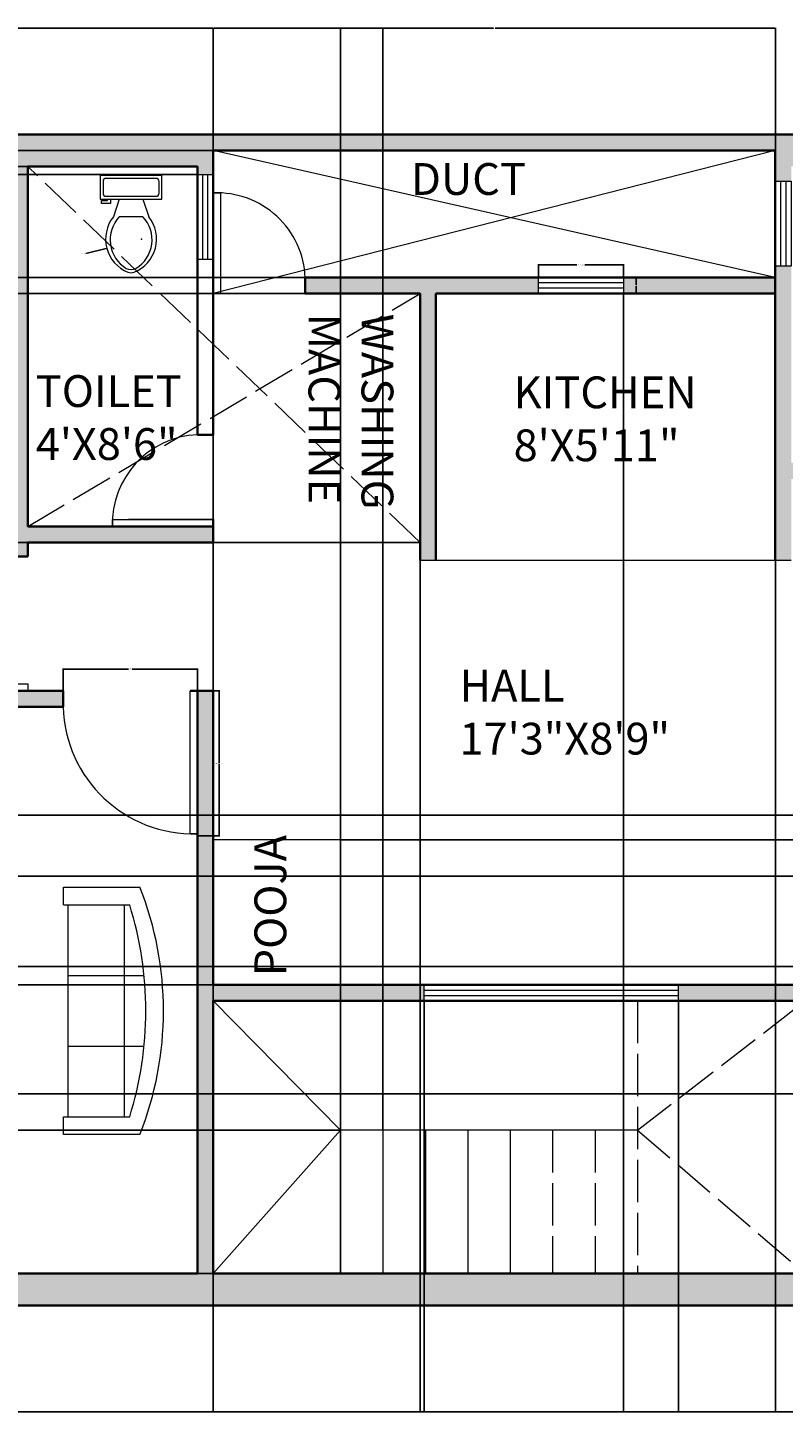
# Model space of a CAD drawing. Units: feet. Extents: x 1699 to 2359, y 1819 to 2211.
# Tile 2 of 4: x 1903 to 2117, y 1819 to 2211. Entities that reach past the tile are written whole.
import ezdxf

# ---------------------------------------------------------------- set-up
doc = ezdxf.new("R2010")
doc.units = ezdxf.units.FT
doc.linetypes.add('ACAD_ISO02W100', pattern=[15, 12, -3])
for name, color, linetype, lineweight in [('A-ANNO-DIMS', 2, 'Continuous', 18), ('A-ANNO-TEXT', 7, 'Continuous', 18), ('A-AREA-IDEN', 7, 'Continuous', 18), ('A-DOOR', 4, 'Continuous', 18), ('A-FLOR', 7, 'Continuous', 18), ('A-FLOR-FIXT', 9, 'Continuous', 18), ('A-FLOR-OVHD', 8, 'ACAD_ISO02W100', 13), ('A-FLOR-STRS', 7, 'Continuous', 18), ('A-FLOR-STRS-OVHD', 8, 'ACAD_ISO02W100', 13), ('A-FURN', 8, 'Continuous', 18), ('A-GLAZ', 3, 'Continuous', 18), ('A-WALL', 7, 'Continuous', 35), ('A-WALL-PATT', 1, 'Continuous', 13)]:
    doc.layers.add(name, color=color, linetype=linetype, lineweight=lineweight)
doc.styles.get("Standard").update_dxf_attribs({"font": 'arial.ttf'})
doc.dimstyles.get("Standard").update_dxf_attribs({"dimtxt": 0.18, "dimasz": 0.18, "dimexe": 0.18, "dimexo": 0.0625, "dimgap": 0.09, "dimtad": 0, "dimtih": 1, "dimtoh": 1, "dimdec": 4, "dimzin": 0, "dimdsep": 46, "dimtxsty": 'Standard', "dimcen": 0.09, "dimadec": 0, "dimazin": 0, "dimtfac": 1, "dimtdec": 4, "dimtofl": 0, "dimtmove": 0, "dimatfit": 3, "dimfxl": 1, "dimtolj": 1, "dimtzin": 0, "dimarcsym": 0})

# ---------------------------------------------------------------- blocks, each defined once
blk = doc.blocks.new('Toilet - top')
for p, q in [((9.5, -6), (9.5, -2)), ((-10, -8.5), (-8, -8.5)), ((-10, -9.5), (-10, -8.5)), ((-8, -8.5), (-8, -8)), ((-7, -8), (-7, -9.5)), ((-4, -8), (-6, -14)), ((4, -8), (6, -14)), ((-7, -9.5), (-10, -9.5)), ((4, -14), (-4, -14))]:
    blk.add_line(p, q)
blk.add_lwpolyline([(10.5, -8), (10.5, 0), (-10.5, 0), (-10.5, -8)], close=True)
for points in [[(-9.5, -2), (-9.5, -6)], [(8.5, -1), (-8.5, -1)], [(-8.5, -7), (8.5, -7)]]:
    blk.add_lwpolyline(points)
for centre, radius, start, end in [((-8.62, -1.88), 0.884, 81.8699, 188.1301), ((8.62, -1.88), 0.884, 351.8699, 98.1301), ((-8.62, -6.12), 0.884, 171.8699, 278.1301), ((8.62, -6.12), 0.884, 261.8699, 8.1301), ((3.52, -21.58), 12.17, 141.4691, 247.9714), ((4.2, -21.82), 11.33, 136.3677, 238.9468), ((-3.52, -21.58), 12.17, 292.0284, 38.5307), ((-4.2, -21.82), 11.33, 301.053, 43.6321), ((0, -27.88), 4, 245.7318, 294.2682), ((0, -29), 4, 254.8605, 285.1395)]:
    blk.add_arc(centre, radius, start, end)
blk = doc.blocks.new('Sofa - Roundback 7 ft.')
for p, q in [((-12.00002, -32.4421), (-12.00003, -6.5971)), ((11.99997, -32.4421), (11.99998, -6.5971)), ((-36.000027, -34), (-36.000027, -11.4696)), ((-35.999844, -13.3819), (35.9998, -13.3819)), ((35.99998, -34), (35.99998, -11.4696)), ((-36.000027, -32.4421), (35.99998, -32.4421))]:
    blk.add_line(p, q)
for points in [[(-36.000027, -34), (-42.000027, -34), (-42.000027, -8)], [(41.99998, -8), (41.99998, -34), (35.99998, -34)]]:
    blk.add_lwpolyline(points)
for centre, radius, start, end in [((0, -114.25), 114.25, 68.43141, 111.5686), ((-0.00001, -127.1968), 121.1968, 72.72033, 107.2797)]:
    blk.add_arc(centre, radius, start, end)
blk = doc.blocks.new('WIN-24-PARTITION')
for p, q in [((0, 24), (4.5, 24)), ((0, 0), (0, 24)), ((1.5, 0), (1.5, 24)), ((3, 0), (3, 24)), ((4.5, 24), (4.5, 0)), ((4.5, 0), (0, 0))]:
    blk.add_line(p, q)
blk = doc.blocks.new('DOOR-SWING-36')
for p, q in [((0.01, 0), (0.01, 2)), ((0.01, 2), (40.51, 2)), ((36.01, 0), (0.01, 0))]:
    blk.add_line(p, q)
blk.add_arc((37.01, 1), 37.01, 91.5482, 181.5482)
blk = doc.blocks.new('DOOR-SWING-24')
for p, q in [((0.02, 0), (0.02, 2)), ((0.02, 2), (28.52, 2)), ((24.02, 0), (0.02, 0))]:
    blk.add_line(p, q)
blk.add_arc((25.02, 1), 25.02, 92.2906, 182.2906)
blk = doc.blocks.new('*D16')
at = {"layer": 'A-ANNO-DIMS', "color": 0, "lineweight": -2, "transparency": 16777216}
for p, q in [((2047.43, 2139.91), (2047.43, 2143.63)), ((2047.61, 2143.45), (2058.31, 2143.45)), ((2071.25, 2143.45), (2060.55, 2143.45)), ((2071.43, 2139.91), (2071.43, 2143.63))]:
    blk.add_line(p, q, dxfattribs=at)
at = {"layer": 'A-ANNO-DIMS', "color": 0, "transparency": 16777216}
for points in [[(2047.61, 2143.48), (2047.61, 2143.42), (2047.43, 2143.45)], [(2071.25, 2143.48), (2071.25, 2143.42), (2071.43, 2143.45)]]:
    blk.add_solid(points, dxfattribs=at)
at = {"layer": 'Defpoints', "color": 0, "transparency": 16777216}
for p in [(2047.43, 2143.45), (2047.43, 2139.85), (2071.43, 2139.85)]:
    blk.add_point(p, dxfattribs=at)
at = {"layer": 'A-ANNO-DIMS', "color": 0, "transparency": 16777216, "insert": (2059.43, 2143.45), "char_height": 0.18, "attachment_point": 5}
blk.add_mtext('\\A1;WINDOW 24 TYP.', dxfattribs=at)
blk = doc.blocks.new('*D17')
at = {"layer": 'A-ANNO-DIMS', "color": 0, "lineweight": -2, "transparency": 16777216}
for p, q in [((2071.49, 2139.85), (2075.21, 2139.85)), ((2075.03, 2139.67), (2075.03, 2137.78)), ((2075.03, 2135.53), (2075.03, 2137.42)), ((2071.49, 2135.35), (2075.21, 2135.35))]:
    blk.add_line(p, q, dxfattribs=at)
at = {"layer": 'A-ANNO-DIMS', "color": 0, "transparency": 16777216}
for points in [[(2075, 2139.67), (2075.06, 2139.67), (2075.03, 2139.85)], [(2075, 2135.53), (2075.06, 2135.53), (2075.03, 2135.35)]]:
    blk.add_solid(points, dxfattribs=at)
at = {"layer": 'Defpoints', "color": 0, "transparency": 16777216}
for p in [(2071.43, 2139.85), (2075.03, 2139.85), (2071.43, 2135.35)]:
    blk.add_point(p, dxfattribs=at)
at = {"layer": 'A-ANNO-DIMS', "color": 0, "transparency": 16777216, "insert": (2075.03, 2137.6), "char_height": 0.18, "attachment_point": 5}
blk.add_mtext('\\A1;5 TYP.', dxfattribs=at)
blk = doc.blocks.new('*D20')
at = {"layer": 'A-ANNO-DIMS', "color": 0, "lineweight": -2, "transparency": 16777216}
for p, q in [((1950.99, 2022.85), (1957.26, 2022.85)), ((1957.08, 2022.67), (1957.08, 2002.51)), ((1957.08, 1981.98), (1957.08, 2002.14)), ((1950.99, 1981.8), (1957.26, 1981.8))]:
    blk.add_line(p, q, dxfattribs=at)
at = {"layer": 'A-ANNO-DIMS', "color": 0, "transparency": 16777216}
for points in [[(1957.05, 2022.67), (1957.11, 2022.67), (1957.08, 2022.85)], [(1957.05, 1981.98), (1957.11, 1981.98), (1957.08, 1981.8)]]:
    blk.add_solid(points, dxfattribs=at)
at = {"layer": 'Defpoints', "color": 0, "transparency": 16777216}
for p in [(1950.93, 2022.85), (1957.08, 2022.85), (1950.93, 1981.8)]:
    blk.add_point(p, dxfattribs=at)
at = {"layer": 'A-ANNO-DIMS', "color": 0, "transparency": 16777216, "insert": (1957.08, 2002.32), "char_height": 0.18, "attachment_point": 5}
blk.add_mtext('\\A1;DOOR D2 41 TYP.', dxfattribs=at)
blk = doc.blocks.new('*D21')
at = {"layer": 'A-ANNO-DIMS', "color": 0, "lineweight": -2, "transparency": 16777216}
for p, q in [((1912.93, 2022.91), (1912.93, 2029.19)), ((1913.11, 2029.01), (1931.4, 2029.01)), ((1950.75, 2029.01), (1932.45, 2029.01)), ((1950.93, 2022.91), (1950.93, 2029.19))]:
    blk.add_line(p, q, dxfattribs=at)
at = {"layer": 'A-ANNO-DIMS', "color": 0, "transparency": 16777216}
for points in [[(1913.11, 2029.04), (1913.11, 2028.98), (1912.93, 2029.01)], [(1950.75, 2029.04), (1950.75, 2028.98), (1950.93, 2029.01)]]:
    blk.add_solid(points, dxfattribs=at)
at = {"layer": 'Defpoints', "color": 0, "transparency": 16777216}
for p in [(1912.93, 2029.01), (1912.93, 2022.85), (1950.93, 2022.85)]:
    blk.add_point(p, dxfattribs=at)
at = {"layer": 'A-ANNO-DIMS', "color": 0, "transparency": 16777216, "insert": (1931.93, 2029.01), "char_height": 0.18, "attachment_point": 5}
blk.add_mtext('\\A1;38 TYP.', dxfattribs=at)
blk = doc.blocks.new('*D23')
at = {"layer": 'A-ANNO-DIMS', "color": 0, "lineweight": -2, "transparency": 16777216}
for p, q in [((1955.43, 1857.79), (1955.43, 1818.57)), ((2180.43, 1857.79), (2180.43, 1818.57)), ((1955.61, 1818.75), (2067.64, 1818.75)), ((2180.25, 1818.75), (2068.22, 1818.75))]:
    blk.add_line(p, q, dxfattribs=at)
at = {"layer": 'A-ANNO-DIMS', "color": 0, "transparency": 16777216}
for points in [[(1955.61, 1818.78), (1955.61, 1818.72), (1955.43, 1818.75)], [(2180.25, 1818.78), (2180.25, 1818.72), (2180.43, 1818.75)]]:
    blk.add_solid(points, dxfattribs=at)
at = {"layer": 'Defpoints', "color": 0, "transparency": 16777216}
for p in [(1955.43, 1857.85), (2180.43, 1857.85), (2180.43, 1818.75)]:
    blk.add_point(p, dxfattribs=at)
at = {"layer": 'A-ANNO-DIMS', "color": 0, "transparency": 16777216, "insert": (2067.93, 1818.75), "char_height": 0.18, "attachment_point": 5}
blk.add_mtext('\\A1;225', dxfattribs=at)
blk = doc.blocks.new('*D24')
at = {"layer": 'A-ANNO-DIMS', "color": 0, "lineweight": -2, "transparency": 16777216}
for p, q in [((1955.49, 1935.08), (2359.21, 1935.08)), ((2359.03, 1934.9), (2359.03, 1896.65)), ((2359.03, 1858.03), (2359.03, 1896.28)), ((1955.49, 1857.85), (2359.21, 1857.85))]:
    blk.add_line(p, q, dxfattribs=at)
at = {"layer": 'A-ANNO-DIMS', "color": 0, "transparency": 16777216}
for points in [[(2359, 1934.9), (2359.06, 1934.9), (2359.03, 1935.08)], [(2359, 1858.03), (2359.06, 1858.03), (2359.03, 1857.85)]]:
    blk.add_solid(points, dxfattribs=at)
at = {"layer": 'Defpoints', "color": 0, "transparency": 16777216}
for p in [(1955.43, 1935.08), (2359.03, 1935.08), (1955.43, 1857.85)]:
    blk.add_point(p, dxfattribs=at)
at = {"layer": 'A-ANNO-DIMS', "color": 0, "transparency": 16777216, "insert": (2359.03, 1896.46), "char_height": 0.18, "attachment_point": 5}
blk.add_mtext('\\A1;77.23', dxfattribs=at)
blk = doc.blocks.new('*D26')
at = {"layer": 'A-ANNO-DIMS', "color": 0, "lineweight": -2, "transparency": 16777216}
for p, q in [((1955.43, 2175.91), (1955.43, 2210.63)), ((1955.61, 2210.45), (2034.65, 2210.45)), ((2114.25, 2210.45), (2035.21, 2210.45)), ((2114.43, 2175.91), (2114.43, 2210.63))]:
    blk.add_line(p, q, dxfattribs=at)
at = {"layer": 'A-ANNO-DIMS', "color": 0, "transparency": 16777216}
for points in [[(1955.61, 2210.48), (1955.61, 2210.42), (1955.43, 2210.45)], [(2114.25, 2210.48), (2114.25, 2210.42), (2114.43, 2210.45)]]:
    blk.add_solid(points, dxfattribs=at)
at = {"layer": 'Defpoints', "color": 0, "transparency": 16777216}
for p in [(2114.43, 2210.45), (1955.43, 2175.85), (2114.43, 2175.85)]:
    blk.add_point(p, dxfattribs=at)
at = {"layer": 'A-ANNO-DIMS', "color": 0, "transparency": 16777216, "insert": (2034.93, 2210.45), "char_height": 0.18, "attachment_point": 5}
blk.add_mtext('\\A1;159', dxfattribs=at)
blk = doc.blocks.new('*D27')
at = {"layer": 'A-ANNO-DIMS', "color": 0, "lineweight": -2, "transparency": 16777216}
for p, q in [((2114.36, 2175.85), (1699.15, 2175.85)), ((1699.33, 2175.67), (1699.33, 2158.03)), ((1699.33, 2140.03), (1699.33, 2157.67)), ((2114.36, 2139.85), (1699.15, 2139.85))]:
    blk.add_line(p, q, dxfattribs=at)
at = {"layer": 'A-ANNO-DIMS', "color": 0, "transparency": 16777216}
for points in [[(1699.3, 2175.67), (1699.36, 2175.67), (1699.33, 2175.85)], [(1699.3, 2140.03), (1699.36, 2140.03), (1699.33, 2139.85)]]:
    blk.add_solid(points, dxfattribs=at)
at = {"layer": 'Defpoints', "color": 0, "transparency": 16777216}
for p in [(2114.43, 2175.85), (1699.33, 2139.85), (2114.43, 2139.85)]:
    blk.add_point(p, dxfattribs=at)
at = {"layer": 'A-ANNO-DIMS', "color": 0, "transparency": 16777216, "insert": (1699.33, 2157.85), "char_height": 0.18, "attachment_point": 5}
blk.add_mtext('\\A1;36', dxfattribs=at)
blk = doc.blocks.new('*D30')
at = {"layer": 'A-ANNO-DIMS', "color": 0, "lineweight": -2, "transparency": 16777216}
for p, q in [((1955.43, 1935.02), (1955.43, 1818.57)), ((2015.05, 1935.02), (2015.05, 1818.57)), ((1955.61, 1818.75), (1984.85, 1818.75)), ((2014.87, 1818.75), (1985.63, 1818.75))]:
    blk.add_line(p, q, dxfattribs=at)
at = {"layer": 'A-ANNO-DIMS', "color": 0, "transparency": 16777216}
for points in [[(1955.61, 1818.78), (1955.61, 1818.72), (1955.43, 1818.75)], [(2014.87, 1818.78), (2014.87, 1818.72), (2015.05, 1818.75)]]:
    blk.add_solid(points, dxfattribs=at)
at = {"layer": 'Defpoints', "color": 0, "transparency": 16777216}
for p in [(1955.43, 1935.08), (2015.05, 1935.08), (2015.05, 1818.75)]:
    blk.add_point(p, dxfattribs=at)
at = {"layer": 'A-ANNO-DIMS', "color": 0, "transparency": 16777216, "insert": (1985.24, 1818.75), "char_height": 0.18, "attachment_point": 5}
blk.add_mtext('\\A1;59.63', dxfattribs=at)
blk = doc.blocks.new('*D31')
at = {"layer": 'A-ANNO-DIMS', "color": 0, "lineweight": -2, "transparency": 16777216}
for p, q in [((2015.05, 1935.02), (2015.05, 1818.57)), ((2087.05, 1935.02), (2087.05, 1818.57)), ((2015.23, 1818.75), (2050.84, 1818.75)), ((2086.87, 1818.75), (2051.27, 1818.75))]:
    blk.add_line(p, q, dxfattribs=at)
at = {"layer": 'A-ANNO-DIMS', "color": 0, "transparency": 16777216}
for points in [[(2015.23, 1818.78), (2015.23, 1818.72), (2015.05, 1818.75)], [(2086.87, 1818.78), (2086.87, 1818.72), (2087.05, 1818.75)]]:
    blk.add_solid(points, dxfattribs=at)
at = {"layer": 'Defpoints', "color": 0, "transparency": 16777216}
for p in [(2015.05, 1935.08), (2087.05, 1935.08), (2087.05, 1818.75)]:
    blk.add_point(p, dxfattribs=at)
at = {"layer": 'A-ANNO-DIMS', "color": 0, "transparency": 16777216, "insert": (2051.05, 1818.75), "char_height": 0.18, "attachment_point": 5}
blk.add_mtext('\\A1;72', dxfattribs=at)
blk = doc.blocks.new('*D32')
at = {"layer": 'A-ANNO-DIMS', "color": 0, "lineweight": -2, "transparency": 16777216}
for p, q in [((1955.43, 1980.78), (1955.43, 2210.63)), ((1955.61, 2210.45), (1973.21, 2210.45)), ((1991.25, 2210.45), (1973.65, 2210.45)), ((1991.43, 1980.78), (1991.43, 2210.63))]:
    blk.add_line(p, q, dxfattribs=at)
at = {"layer": 'A-ANNO-DIMS', "color": 0, "transparency": 16777216}
for points in [[(1955.61, 2210.48), (1955.61, 2210.42), (1955.43, 2210.45)], [(1991.25, 2210.48), (1991.25, 2210.42), (1991.43, 2210.45)]]:
    blk.add_solid(points, dxfattribs=at)
at = {"layer": 'Defpoints', "color": 0, "transparency": 16777216}
for p in [(1991.43, 2210.45), (1955.43, 1980.71), (1991.43, 1980.71)]:
    blk.add_point(p, dxfattribs=at)
at = {"layer": 'A-ANNO-DIMS', "color": 0, "transparency": 16777216, "insert": (1973.43, 2210.45), "char_height": 0.18, "attachment_point": 5}
blk.add_mtext('\\A1;36', dxfattribs=at)
blk = doc.blocks.new('*D33')
at = {"layer": 'A-ANNO-DIMS', "color": 0, "lineweight": -2, "transparency": 16777216}
for p, q in [((1991.49, 1980.71), (2359.21, 1980.71)), ((2359.03, 1980.53), (2359.03, 1960.33)), ((2359.03, 1939.76), (2359.03, 1959.97)), ((1955.49, 1939.58), (2359.21, 1939.58))]:
    blk.add_line(p, q, dxfattribs=at)
at = {"layer": 'A-ANNO-DIMS', "color": 0, "transparency": 16777216}
for points in [[(2359, 1980.53), (2359.06, 1980.53), (2359.03, 1980.71)], [(2359, 1939.76), (2359.06, 1939.76), (2359.03, 1939.58)]]:
    blk.add_solid(points, dxfattribs=at)
at = {"layer": 'Defpoints', "color": 0, "transparency": 16777216}
for p in [(1991.43, 1980.71), (1955.43, 1939.58), (2359.03, 1939.58)]:
    blk.add_point(p, dxfattribs=at)
at = {"layer": 'A-ANNO-DIMS', "color": 0, "transparency": 16777216, "insert": (2359.03, 1960.15), "char_height": 0.18, "attachment_point": 5}
blk.add_mtext('\\A1;41.14', dxfattribs=at)
blk = doc.blocks.new('*D38')
at = {"layer": 'A-ANNO-DIMS', "color": 0, "lineweight": -2, "transparency": 16777216}
for p, q in [((1784.49, 1944.78), (2359.21, 1944.78)), ((2359.03, 1944.6), (2359.03, 1926.96)), ((2359.03, 1908.96), (2359.03, 1926.6)), ((1784.49, 1908.78), (2359.21, 1908.78))]:
    blk.add_line(p, q, dxfattribs=at)
at = {"layer": 'A-ANNO-DIMS', "color": 0, "transparency": 16777216}
for points in [[(2359, 1944.6), (2359.06, 1944.6), (2359.03, 1944.78)], [(2359, 1908.96), (2359.06, 1908.96), (2359.03, 1908.78)]]:
    blk.add_solid(points, dxfattribs=at)
at = {"layer": 'Defpoints', "color": 0, "transparency": 16777216}
for p in [(1784.43, 1944.78), (2359.03, 1944.78), (1784.43, 1908.78)]:
    blk.add_point(p, dxfattribs=at)
at = {"layer": 'A-ANNO-DIMS', "color": 0, "transparency": 16777216, "insert": (2359.03, 1926.78), "char_height": 0.18, "attachment_point": 5}
blk.add_mtext('\\A1;36', dxfattribs=at)
blk = doc.blocks.new('*D39')
at = {"layer": 'A-ANNO-DIMS', "color": 0, "lineweight": -2, "transparency": 16777216}
for p, q in [((1784.49, 1987.61), (2359.21, 1987.61)), ((2359.03, 1987.43), (2359.03, 1966.38)), ((2359.03, 1944.96), (2359.03, 1966.02)), ((1784.49, 1944.78), (2359.21, 1944.78))]:
    blk.add_line(p, q, dxfattribs=at)
at = {"layer": 'A-ANNO-DIMS', "color": 0, "transparency": 16777216}
for points in [[(2359, 1987.43), (2359.06, 1987.43), (2359.03, 1987.61)], [(2359, 1944.96), (2359.06, 1944.96), (2359.03, 1944.78)]]:
    blk.add_solid(points, dxfattribs=at)
at = {"layer": 'Defpoints', "color": 0, "transparency": 16777216}
for p in [(1784.43, 1987.61), (2359.03, 1987.61), (1784.43, 1944.78)]:
    blk.add_point(p, dxfattribs=at)
at = {"layer": 'A-ANNO-DIMS', "color": 0, "transparency": 16777216, "insert": (2359.03, 1966.2), "char_height": 0.18, "attachment_point": 5}
blk.add_mtext('\\A1;42.83', dxfattribs=at)
blk = doc.blocks.new('*D40')
at = {"layer": 'A-ANNO-DIMS', "color": 0, "lineweight": -2, "transparency": 16777216}
for p, q in [((1729.43, 1848.79), (1729.43, 1818.57)), ((2328.93, 1848.79), (2328.93, 1818.57)), ((1729.61, 1818.75), (2028.78, 1818.75)), ((2328.75, 1818.75), (2029.57, 1818.75))]:
    blk.add_line(p, q, dxfattribs=at)
at = {"layer": 'A-ANNO-DIMS', "color": 0, "transparency": 16777216}
for points in [[(1729.61, 1818.78), (1729.61, 1818.72), (1729.43, 1818.75)], [(2328.75, 1818.78), (2328.75, 1818.72), (2328.93, 1818.75)]]:
    blk.add_solid(points, dxfattribs=at)
at = {"layer": 'Defpoints', "color": 0, "transparency": 16777216}
for p in [(1729.43, 1848.85), (2328.93, 1848.85), (2328.93, 1818.75)]:
    blk.add_point(p, dxfattribs=at)
at = {"layer": 'A-ANNO-DIMS', "color": 0, "transparency": 16777216, "insert": (2029.18, 1818.75), "char_height": 0.18, "attachment_point": 5}
blk.add_mtext('\\A1;599.5', dxfattribs=at)
blk = doc.blocks.new('*D42')
at = {"layer": 'A-ANNO-DIMS', "color": 0, "lineweight": -2, "transparency": 16777216}
for p, q in [((1991.43, 1898.53), (1991.43, 2210.63)), ((1991.61, 2210.45), (1997.22, 2210.45)), ((2003.25, 2210.45), (1997.64, 2210.45)), ((2003.43, 1898.53), (2003.43, 2210.63))]:
    blk.add_line(p, q, dxfattribs=at)
at = {"layer": 'A-ANNO-DIMS', "color": 0, "transparency": 16777216}
for points in [[(1991.61, 2210.48), (1991.61, 2210.42), (1991.43, 2210.45)], [(2003.25, 2210.48), (2003.25, 2210.42), (2003.43, 2210.45)]]:
    blk.add_solid(points, dxfattribs=at)
at = {"layer": 'Defpoints', "color": 0, "transparency": 16777216}
for p in [(2003.43, 2210.45), (1991.43, 1898.47), (2003.43, 1898.47)]:
    blk.add_point(p, dxfattribs=at)
at = {"layer": 'A-ANNO-DIMS', "color": 0, "transparency": 16777216, "insert": (1997.43, 2210.45), "char_height": 0.18, "attachment_point": 5}
blk.add_mtext('\\A1;12', dxfattribs=at)
blk = doc.blocks.new('*D43')
at = {"layer": 'A-ANNO-DIMS', "color": 0, "lineweight": -2, "transparency": 16777216}
for p, q in [((1991.36, 1898.47), (1699.15, 1898.47)), ((1699.33, 1898.29), (1699.33, 1878.34)), ((1699.33, 1858.03), (1699.33, 1877.98)), ((1991.36, 1857.85), (1699.15, 1857.85))]:
    blk.add_line(p, q, dxfattribs=at)
at = {"layer": 'A-ANNO-DIMS', "color": 0, "transparency": 16777216}
for points in [[(1699.3, 1898.29), (1699.36, 1898.29), (1699.33, 1898.47)], [(1699.3, 1858.03), (1699.36, 1858.03), (1699.33, 1857.85)]]:
    blk.add_solid(points, dxfattribs=at)
at = {"layer": 'Defpoints', "color": 0, "transparency": 16777216}
for p in [(1991.43, 1898.47), (1699.33, 1857.85), (1991.43, 1857.85)]:
    blk.add_point(p, dxfattribs=at)
at = {"layer": 'A-ANNO-DIMS', "color": 0, "transparency": 16777216, "insert": (1699.33, 1878.16), "char_height": 0.18, "attachment_point": 5}
blk.add_mtext('\\A1;40.62', dxfattribs=at)
blk = doc.blocks.new('*D44')
at = {"layer": 'A-ANNO-DIMS', "color": 0, "lineweight": -2, "transparency": 16777216}
for p, q in [((1955.43, 1857.91), (1955.43, 2210.63)), ((1955.61, 2210.45), (1973.21, 2210.45)), ((1991.25, 2210.45), (1973.65, 2210.45)), ((1991.43, 1857.91), (1991.43, 2210.63))]:
    blk.add_line(p, q, dxfattribs=at)
at = {"layer": 'A-ANNO-DIMS', "color": 0, "transparency": 16777216}
for points in [[(1955.61, 2210.48), (1955.61, 2210.42), (1955.43, 2210.45)], [(1991.25, 2210.48), (1991.25, 2210.42), (1991.43, 2210.45)]]:
    blk.add_solid(points, dxfattribs=at)
at = {"layer": 'Defpoints', "color": 0, "transparency": 16777216}
for p in [(1991.43, 2210.45), (1955.43, 1857.85), (1991.43, 1857.85)]:
    blk.add_point(p, dxfattribs=at)
at = {"layer": 'A-ANNO-DIMS', "color": 0, "transparency": 16777216, "insert": (1973.43, 2210.45), "char_height": 0.18, "attachment_point": 5}
blk.add_mtext('\\A1;36', dxfattribs=at)
blk = doc.blocks.new('*D45')
at = {"layer": 'A-ANNO-DIMS', "color": 0, "lineweight": -2, "transparency": 16777216}
for p, q in [((1955.43, 2064.79), (1955.43, 1818.57)), ((2013.93, 2064.79), (2013.93, 1818.57)), ((1955.61, 1818.75), (1984.35, 1818.75)), ((2013.75, 1818.75), (1985, 1818.75))]:
    blk.add_line(p, q, dxfattribs=at)
at = {"layer": 'A-ANNO-DIMS', "color": 0, "transparency": 16777216}
for points in [[(1955.61, 1818.78), (1955.61, 1818.72), (1955.43, 1818.75)], [(2013.75, 1818.78), (2013.75, 1818.72), (2013.93, 1818.75)]]:
    blk.add_solid(points, dxfattribs=at)
at = {"layer": 'Defpoints', "color": 0, "transparency": 16777216}
for p in [(1955.43, 2064.85), (2013.93, 2064.85), (2013.93, 1818.75)]:
    blk.add_point(p, dxfattribs=at)
at = {"layer": 'A-ANNO-DIMS', "color": 0, "transparency": 16777216, "insert": (1984.68, 1818.75), "char_height": 0.18, "attachment_point": 5}
blk.add_mtext('\\A1;58.5', dxfattribs=at)
blk = doc.blocks.new('*D46')
at = {"layer": 'A-ANNO-DIMS', "color": 0, "lineweight": -2, "transparency": 16777216}
for p, q in [((2013.86, 2135.35), (1699.15, 2135.35)), ((1699.33, 2135.17), (1699.33, 2100.28)), ((1699.33, 2065.03), (1699.33, 2099.92)), ((2013.86, 2064.85), (1699.15, 2064.85))]:
    blk.add_line(p, q, dxfattribs=at)
at = {"layer": 'A-ANNO-DIMS', "color": 0, "transparency": 16777216}
for points in [[(1699.3, 2135.17), (1699.36, 2135.17), (1699.33, 2135.35)], [(1699.3, 2065.03), (1699.36, 2065.03), (1699.33, 2064.85)]]:
    blk.add_solid(points, dxfattribs=at)
at = {"layer": 'Defpoints', "color": 0, "transparency": 16777216}
for p in [(1699.33, 2135.35), (2013.93, 2135.35), (2013.93, 2064.85)]:
    blk.add_point(p, dxfattribs=at)
at = {"layer": 'A-ANNO-DIMS', "color": 0, "transparency": 16777216, "insert": (1699.33, 2100.1), "char_height": 0.18, "attachment_point": 5}
blk.add_mtext('\\A1;70.5', dxfattribs=at)
blk = doc.blocks.new('*D48')
at = {"layer": 'A-ANNO-DIMS', "color": 0, "lineweight": -2, "transparency": 16777216}
for p, q in [((2180.36, 1970.41), (1699.15, 1970.41)), ((1699.33, 1970.23), (1699.33, 1955.18)), ((1699.33, 1939.76), (1699.33, 1954.81)), ((2180.36, 1939.58), (1699.15, 1939.58))]:
    blk.add_line(p, q, dxfattribs=at)
at = {"layer": 'A-ANNO-DIMS', "color": 0, "transparency": 16777216}
for points in [[(1699.3, 1970.23), (1699.36, 1970.23), (1699.33, 1970.41)], [(1699.3, 1939.76), (1699.36, 1939.76), (1699.33, 1939.58)]]:
    blk.add_solid(points, dxfattribs=at)
at = {"layer": 'Defpoints', "color": 0, "transparency": 16777216}
for p in [(1699.33, 1970.41), (2180.43, 1970.41), (2180.43, 1939.58)]:
    blk.add_point(p, dxfattribs=at)
at = {"layer": 'A-ANNO-DIMS', "color": 0, "transparency": 16777216, "insert": (1699.33, 1954.99), "char_height": 0.18, "attachment_point": 5}
blk.add_mtext('\\A1;30.833', dxfattribs=at)
blk = doc.blocks.new('*D49')
at = {"layer": 'A-ANNO-DIMS', "color": 0, "lineweight": -2, "transparency": 16777216}
for p, q in [((2071.43, 2135.29), (2071.43, 1818.57)), ((2114.43, 2135.29), (2114.43, 1818.57)), ((2071.61, 1818.75), (2092.71, 1818.75)), ((2114.25, 1818.75), (2093.15, 1818.75))]:
    blk.add_line(p, q, dxfattribs=at)
at = {"layer": 'A-ANNO-DIMS', "color": 0, "transparency": 16777216}
for points in [[(2071.61, 1818.78), (2071.61, 1818.72), (2071.43, 1818.75)], [(2114.25, 1818.78), (2114.25, 1818.72), (2114.43, 1818.75)]]:
    blk.add_solid(points, dxfattribs=at)
at = {"layer": 'Defpoints', "color": 0, "transparency": 16777216}
for p in [(2071.43, 2135.35), (2114.43, 2135.35), (2114.43, 1818.75)]:
    blk.add_point(p, dxfattribs=at)
at = {"layer": 'A-ANNO-DIMS', "color": 0, "transparency": 16777216, "insert": (2092.93, 1818.75), "char_height": 0.18, "attachment_point": 5}
blk.add_mtext('\\A1;43', dxfattribs=at)
blk = doc.blocks.new('*D50')
at = {"layer": 'A-ANNO-DIMS', "color": 0, "lineweight": -2, "transparency": 16777216}
for p, q in [((1950.86, 2171.35), (1699.15, 2171.35)), ((1950.86, 2169.04), (1699.15, 2169.04)), ((1699.33, 2171.17), (1699.33, 2170.38)), ((1699.33, 2169.22), (1699.33, 2170.01))]:
    blk.add_line(p, q, dxfattribs=at)
at = {"layer": 'A-ANNO-DIMS', "color": 0, "transparency": 16777216}
for points in [[(1699.3, 2171.17), (1699.36, 2171.17), (1699.33, 2171.35)], [(1699.3, 2169.22), (1699.36, 2169.22), (1699.33, 2169.04)]]:
    blk.add_solid(points, dxfattribs=at)
at = {"layer": 'Defpoints', "color": 0, "transparency": 16777216}
for p in [(1699.33, 2169.04), (1950.93, 2171.35), (1950.93, 2169.04)]:
    blk.add_point(p, dxfattribs=at)
at = {"layer": 'A-ANNO-DIMS', "color": 0, "transparency": 16777216, "insert": (1699.33, 2170.19), "char_height": 0.18, "attachment_point": 5}
blk.add_mtext('\\A1;2.312', dxfattribs=at)
blk = doc.blocks.new('*D52')
at = {"layer": 'A-ANNO-DIMS', "color": 0, "lineweight": -2, "transparency": 16777216}
for p, q in [((1729.43, 2180.41), (1729.43, 2210.63)), ((1729.61, 2210.45), (1842.14, 2210.45)), ((1955.25, 2210.45), (1842.72, 2210.45)), ((1955.43, 2175.91), (1955.43, 2210.63))]:
    blk.add_line(p, q, dxfattribs=at)
at = {"layer": 'A-ANNO-DIMS', "color": 0, "transparency": 16777216}
for points in [[(1729.61, 2210.48), (1729.61, 2210.42), (1729.43, 2210.45)], [(1955.25, 2210.48), (1955.25, 2210.42), (1955.43, 2210.45)]]:
    blk.add_solid(points, dxfattribs=at)
at = {"layer": 'Defpoints', "color": 0, "transparency": 16777216}
for p in [(1955.43, 2210.45), (1729.43, 2180.35), (1955.43, 2175.85)]:
    blk.add_point(p, dxfattribs=at)
at = {"layer": 'A-ANNO-DIMS', "color": 0, "transparency": 16777216, "insert": (1842.43, 2210.45), "char_height": 0.18, "attachment_point": 5}
blk.add_mtext('\\A1;226', dxfattribs=at)
blk = doc.blocks.new('*D63')
at = {"layer": 'A-ANNO-DIMS', "color": 0, "lineweight": -2, "transparency": 16777216}
for p, q in [((1935, 2150.78), (1935.18, 2150.78)), ((1935.09, 2150.69), (1935.09, 2150.87)), ((1919.4, 2146.65), (1925.11, 2148.15))]:
    blk.add_line(p, q, dxfattribs=at)
at = {"layer": 'A-ANNO-DIMS', "color": 0, "transparency": 16777216}
blk.add_solid([(1925.1, 2148.18), (1925.12, 2148.13), (1925.29, 2148.2)], dxfattribs=at)
at = {"layer": 'Defpoints', "color": 0, "transparency": 16777216}
for p in [(1935.09, 2150.78), (1925.29, 2148.2)]:
    blk.add_point(p, dxfattribs=at)
at = {"layer": 'A-ANNO-DIMS', "color": 0, "transparency": 16777216, "insert": (1918.73, 2146.65), "char_height": 0.18, "attachment_point": 5}
blk.add_mtext('\\A1;4X R10.14', dxfattribs=at)

msp = doc.modelspace()

# ---------------------------------------------------------------- hatches: boundary and pattern name
at = {"layer": 'A-WALL-PATT'}
h = msp.add_hatch(color=256, dxfattribs=at)
h.dxf.hatch_style = 1
h.paths.add_polyline_path([(2180.4267, 1853.3494), (2180.4267, 1857.8494), (1955.4267, 1857.8494), (1955.4267, 1935.0782), (1991.4267, 1935.0782), (1991.4267, 1939.5782), (1955.4267, 1939.5782), (1955.4267, 2022.8494), (1950.9267, 2022.8494), (1950.9267, 1857.8494), (1784.4267, 1857.8494), (1784.4267, 1908.7829), (1775.4267, 1908.7829), (1775.4267, 1853.3494), (1733.9267, 1853.3494), (1733.9267, 2018.3494), (1775.4267, 2018.3494), (1775.4267, 2022.8494), (1738.4267, 2022.8494), (1738.4267, 2171.3494), (1898.4267, 2171.3494), (1898.4267, 2060.8494), (1902.9267, 2060.8494), (1902.9267, 2064.8494), (1955.4267, 2064.8494), (1955.4267, 2069.3494), (1902.9267, 2069.3494), (1902.9267, 2171.3494), (1950.9267, 2171.3494), (1950.9267, 2169.0373), (1955.4267, 2169.0373), (1955.4267, 2175.8494), (2114.4267, 2175.8494), (2114.4267, 2167.1408), (2118.9267, 2167.1408), (2118.9267, 2171.3494), (2166.9267, 2171.3494), (2166.9267, 2113.3494), (2171.4267, 2113.3494), (2171.4267, 2171.3494), (2319.9267, 2171.3494), (2319.9267, 2132.5785), (2328.9267, 2132.5785), (2328.9267, 2180.3494), (2309.4267, 2180.3494), (1729.4267, 2180.3494), (1729.4267, 1848.8494), (2180.4267, 1848.8494)])
h.paths.add_polyline_path([(1784.4267, 1987.6139), (1775.4267, 1987.6139), (1775.4267, 1944.7829), (1784.4267, 1944.7829)], flags=17)
h.paths.add_polyline_path([(1912.9267, 2022.8494), (1775.4267, 2022.8494), (1775.4267, 2013.6139), (1784.4267, 2013.6139), (1784.4267, 2018.3494), (1912.9267, 2018.3494)], flags=17)
h.paths.add_polyline_path([(2018.4267, 2135.3494), (2047.4307, 2135.3494), (2047.4307, 2139.8494), (1981.4267, 2139.8494), (1981.4267, 2135.3494), (2013.9267, 2135.3494), (2013.9267, 2059.8494), (2018.4267, 2059.8494)], flags=17)
h.paths.add_polyline_path([(2114.4267, 2139.8494), (2071.4307, 2139.8494), (2071.4307, 2135.3494), (2114.4267, 2135.3494)], flags=17)
h.paths.add_polyline_path([(2118.9267, 2143.1408), (2114.4267, 2143.1408), (2114.4267, 2059.8494), (2118.9267, 2059.8494), (2118.9267, 2082.8494), (2184.631, 2082.8494), (2184.631, 2087.3494), (2118.9267, 2087.3494)], flags=17)
h.paths.add_polyline_path([(2328.9267, 2084.5785), (2319.9267, 2084.5785), (2319.9267, 2022.8494), (2232.7955, 2022.8494), (2232.7955, 2013.3494), (2319.9267, 2013.3494), (2319.9267, 1998.3723), (2328.9267, 1998.3723)], flags=17)
h.paths.add_polyline_path([(2180.4267, 2043.5261), (2171.4267, 2043.5261), (2171.4267, 2006.4114), (2180.4267, 2006.4114)], flags=17)
h.paths.add_polyline_path([(2015.0526, 1939.5782), (1991.4267, 1939.5782), (1991.4267, 1935.0782), (2015.0526, 1935.0782)], flags=17)
h.paths.add_polyline_path([(2180.4267, 1939.5782), (2087.0526, 1939.5782), (2087.0526, 1935.0782), (2180.4267, 1935.0782)], flags=17)
h.paths.add_polyline_path([(2328.9267, 1868.1839), (2319.9267, 1868.1839), (2319.9267, 1853.3494), (2180.4267, 1853.3494), (2180.4267, 1848.8494), (2328.9267, 1848.8494)], flags=17)

# ---------------------------------------------------------------- linework, layer by layer
at = {"layer": 'A-DOOR'}
for p, q in [((1955.4267, 2135.3494), (1957.4267, 2135.3494)), ((1955.4267, 2071.3494), (1931.4267, 2071.3494)), ((1931.4267, 2071.3494), (1955.4267, 2071.3494)), ((1902.9267, 2024.8494), (1902.9267, 2022.8494))]:
    msp.add_line(p, q, dxfattribs=at)
at = {"layer": 'A-FLOR'}
for p, q in [((2114.4267, 2139.8494), (1955.4267, 2175.8494)), ((2114.4267, 2175.8494), (1955.4267, 2135.3494)), ((1955.4267, 2064.8494), (2013.9267, 2064.8494)), ((2013.9267, 2059.8494), (2118.9267, 2059.8494)), ((1991.4267, 1980.7142), (1955.4267, 1980.7142)), ((1991.4267, 1935.0782), (1991.4267, 1980.7142))]:
    msp.add_line(p, q, dxfattribs=at)
at = {"layer": 'A-FLOR-OVHD'}
for p, q in [((2013.9267, 2064.8494), (1902.9267, 2171.3494)), ((1902.9267, 2069.3494), (2013.9267, 2135.3494))]:
    msp.add_line(p, q, dxfattribs=at)
at = {"layer": 'A-FLOR-STRS'}
for p, q in [((1991.4267, 1898.4702), (1955.4267, 1935.0782)), ((1991.4267, 1935.0782), (1991.4267, 1857.8494)), ((1991.4267, 1898.4702), (1955.4267, 1857.8494)), ((2075.4267, 1898.4702), (1991.4267, 1898.4702)), ((2003.4267, 1898.4702), (2003.4267, 1857.8494)), ((2015.4267, 1898.4702), (2015.4267, 1857.8494)), ((2027.4267, 1898.4702), (2027.4267, 1857.8494)), ((2039.4267, 1898.4702), (2039.4267, 1857.8494))]:
    msp.add_line(p, q, dxfattribs=at)
at = {"layer": 'A-FLOR-STRS-OVHD'}
for p, q in [((2075.4267, 1935.0782), (2075.4267, 1857.8494)), ((2075.4267, 1898.4702), (2122.862, 1935.0782)), ((2051.4267, 1898.4702), (2051.4267, 1857.8494)), ((2063.4267, 1898.4702), (2063.4267, 1857.8494)), ((2075.4267, 1898.4702), (2122.862, 1857.8494))]:
    msp.add_line(p, q, dxfattribs=at)
at = {"layer": 'A-GLAZ'}
for p, q in [((2015.0526, 1935.0782), (2015.0526, 1939.5782)), ((2087.0526, 1939.5782), (2015.0526, 1939.5782)), ((2015.0526, 1938.0782), (2087.0526, 1938.0782)), ((2087.0526, 1935.0782), (2087.0526, 1939.5782)), ((2015.0526, 1936.5782), (2087.0526, 1936.5782)), ((2015.0526, 1935.0782), (2087.0526, 1935.0782))]:
    msp.add_line(p, q, dxfattribs=at)
at = {"layer": 'A-WALL'}
for p, q in [((1729.4267, 2180.3494), (2309.4267, 2180.3494)), ((1955.4267, 2175.8494), (1955.4267, 2095.3494)), ((1955.4267, 2175.8494), (2114.4267, 2175.8494)), ((2114.4267, 2175.8494), (2114.4267, 2059.8494)), ((1902.9267, 2171.3494), (1902.9267, 2069.3494)), ((1902.9267, 2171.3494), (1950.9267, 2171.3494)), ((1950.9267, 2171.3494), (1950.9267, 2095.3494)), ((1981.4267, 2139.8494), (2114.4267, 2139.8494)), ((1981.4267, 2135.3494), (1981.4267, 2139.8494)), ((1981.4267, 2135.3494), (2013.9267, 2135.3494)), ((2013.9267, 2135.3494), (2013.9267, 2059.8494)), ((2018.4267, 2135.3494), (2018.4267, 2059.8494)), ((2018.4267, 2135.3494), (2114.4267, 2135.3494)), ((1955.4267, 2095.3494), (1950.9267, 2095.3494)), ((1955.4267, 2071.3494), (1955.4267, 2064.8494)), ((1902.9267, 2069.3494), (1955.4267, 2069.3494)), ((1902.9267, 2064.8494), (1955.4267, 2064.8494)), ((1902.9267, 2064.8494), (1902.9267, 2060.8494)), ((1902.9267, 2060.8494), (1898.4267, 2060.8494)), ((1738.4267, 2022.8494), (1912.9267, 2022.8494)), ((1912.9267, 2022.8494), (1912.9267, 2018.3494)), ((1948.9267, 2022.8494), (1955.4267, 2022.8494)), ((1950.9267, 2022.8494), (1950.9267, 1857.8494)), ((1955.4267, 2022.8494), (1955.4267, 1939.5782)), ((1784.4267, 2018.3494), (1912.9267, 2018.3494)), ((1955.4267, 1939.5782), (2180.4267, 1939.5782)), ((1955.4267, 1935.0782), (2180.4267, 1935.0782)), ((1955.4267, 1935.0782), (1955.4267, 1857.8494)), ((1784.4267, 1857.8494), (1950.9267, 1857.8494)), ((1955.4267, 1857.8494), (2180.4267, 1857.8494)), ((1729.4267, 1848.8494), (2328.9267, 1848.8494))]:
    msp.add_line(p, q, dxfattribs=at)

# ---------------------------------------------------------------- block references
at = {"layer": 'A-DOOR'}
for name, p, rotation in [('DOOR-SWING-24', (1955.4263, 2163.868), 269.9999999999995), ('DOOR-SWING-36', (1950.927, 1982.3357), 90.00000000000024)]:
    msp.add_blockref(name, p, dxfattribs=dict(at, rotation=rotation))
for name, p in [('DOOR-SWING-24', (1926.908, 2069.349)), ('DOOR-SWING-36', (1862.413, 2022.849))]:
    msp.add_blockref(name, p, dxfattribs=at)
at = {"layer": 'A-FLOR-FIXT', "xscale": 0.8333333333333331, "yscale": 0.8333333333333331, "zscale": 0.8333333333333331}
msp.add_blockref('Toilet - top', (1932.1616, 2168.7609), dxfattribs=at)
at = {"layer": 'A-FURN', "xscale": 0.8333333333333331, "yscale": 0.8333333333333331, "zscale": 0.8333333333333331, "rotation": 270}
msp.add_blockref('Sofa - Roundback 7 ft.', (1941.3382, 1932.2553), dxfattribs=at)
at = {"layer": 'A-GLAZ'}
msp.add_blockref('WIN-24-PARTITION', (1950.927, 2145.037), dxfattribs=at)
for p, rotation in [((2118.9263, 2167.1411), 180), ((2071.431, 2135.3497), 90.00000000000026)]:
    msp.add_blockref('WIN-24-PARTITION', p, dxfattribs=dict(at, rotation=rotation))

# ---------------------------------------------------------------- texts
at = {"layer": 'A-ANNO-TEXT', "insert": (2006.3642, 2129.6332), "char_height": 9, "attachment_point": 1, "rotation": 270}
msp.add_mtext_dynamic_manual_height_columns('{\\fCambria|b0|i0|c0|p18;WASHING MACHINE}', width=47.451108, gutter_width=12.5, heights=[0], dxfattribs=at)
at = {"layer": 'A-AREA-IDEN', "char_height": 9, "attachment_point": 1}
for s, width, insert in [('{\\fCambria|b0|i0|c0|p18;DUCT}', 54.644204, (2011.3809, 2172.2896)), ('{\\fCambria|b0|i0|c0|p18;TOILET\\P4\'X8\'6"}', 42.504465, (1905.2036, 2112.2388)), ('{\\fCambria|b0|i0|c0|p18;KITCHEN\\P8\'X5\'11"}', 70.116007, (2040.3902, 2111.8741)), ('{\\fCambria|b0|i0|c0|p18;HALL\\P17\'3"X8\'9"}', 85.745118, (2025.0681, 2028.8262))]:
    msp.add_mtext_dynamic_manual_height_columns(s, width=width, gutter_width=12.5, heights=[0], dxfattribs=dict(at, insert=insert))
at = {"layer": 'A-AREA-IDEN', "insert": (1967.0731, 1942.0138), "char_height": 9, "attachment_point": 1, "rotation": 90}
msp.add_mtext_dynamic_manual_height_columns('{\\fCambria|b0|i0|c0|p18;POOJA}', width=27.385, gutter_width=12.5, heights=[0], dxfattribs=at)

# ---------------------------------------------------------------- dimensions: what is measured, and where the dimension line sits
at = {"layer": 'A-ANNO-DIMS'}
for base, p1, p2, override, picture, middle in [((1955.4267, 2210.4494), (1729.4267, 2180.3494), (1955.4267, 2175.8494), {"dimdec": 0, "dimlfac": 1, "dimrnd": 0, "dimzin": 0, "dimdsep": 46, "dimlunit": 2}, '*D52', (1842.4267, 2210.4494)), ((2114.4267, 2210.4494), (1955.4267, 2175.8494), (2114.4267, 2175.8494), {"dimdec": 0, "dimlfac": 1, "dimrnd": 0, "dimzin": 0, "dimdsep": 46, "dimlunit": 2}, '*D26', (2034.9267, 2210.4494)), ((1991.4267, 2210.4494), (1955.4267, 1980.7142), (1991.4267, 1980.7142), {"dimdec": 0, "dimlfac": 1, "dimrnd": 0, "dimzin": 0, "dimdsep": 46, "dimlunit": 2}, '*D32', (1973.4267, 2210.4494)), ((1991.4267, 2210.4494), (1955.4267, 1857.8494), (1991.4267, 1857.8494), {"dimdec": 0, "dimlfac": 1, "dimrnd": 0, "dimzin": 0, "dimdsep": 46, "dimlunit": 2}, '*D44', (1973.4267, 2210.4494)), ((2003.4267, 2210.4494), (1991.4267, 1898.4702), (2003.4267, 1898.4702), {"dimdec": 0, "dimlfac": 1, "dimrnd": 0, "dimzin": 0, "dimdsep": 46, "dimlunit": 2}, '*D42', (1997.4267, 2210.4494)), ((2114.4267, 1818.7494), (2071.4307, 2135.3494), (2114.4267, 2135.3494), {"dimdec": 0, "dimlfac": 1, "dimrnd": 0, "dimzin": 0, "dimdsep": 46, "dimlunit": 2}, '*D49', (2092.9287, 1818.7494)), ((2013.9267, 1818.7494), (1955.4267, 2064.8494), (2013.9267, 2064.8494), {"dimdec": 1, "dimlfac": 1, "dimrnd": 0, "dimzin": 0, "dimdsep": 46, "dimlunit": 2}, '*D45', (1984.6767, 1818.7494)), ((2015.0526, 1818.7494), (1955.4267, 1935.0782), (2015.0526, 1935.0782), {"dimdec": 2, "dimlfac": 1, "dimrnd": 0, "dimzin": 0, "dimdsep": 46, "dimlunit": 2}, '*D30', (1985.2396, 1818.7494)), ((2087.0526, 1818.7494), (2015.0526, 1935.0782), (2087.0526, 1935.0782), {"dimdec": 0, "dimlfac": 1, "dimrnd": 0, "dimzin": 0, "dimdsep": 46, "dimlunit": 2}, '*D31', (2051.0526, 1818.7494)), ((2180.4267, 1818.7494), (1955.4267, 1857.8494), (2180.4267, 1857.8494), {"dimdec": 0, "dimlfac": 1, "dimrnd": 0, "dimzin": 0, "dimdsep": 46, "dimlunit": 2}, '*D23', (2067.9267, 1818.7494)), ((2328.9267, 1818.7494), (1729.4267, 1848.8494), (2328.9267, 1848.8494), {"dimdec": 1, "dimlfac": 1, "dimrnd": 0, "dimzin": 0, "dimdsep": 46, "dimlunit": 2}, '*D40', (2029.1767, 1818.7494))]:
    dim = msp.add_linear_dim(base=base, p1=p1, p2=p2, dimstyle='Standard', override=override, dxfattribs=at)
    dim.commit()
    dim.dimension.update_dxf_attribs({"geometry": picture, "text_midpoint": middle})
for base, p1, p2, override, picture, middle in [((1699.3267, 2139.8494), (2114.4267, 2175.8494), (2114.4267, 2139.8494), {"dimdec": 0, "dimlfac": 1, "dimrnd": 0, "dimzin": 0, "dimdsep": 46, "dimlunit": 2}, '*D27', (1699.3267, 2157.8494)), ((1699.3267, 2169.0373), (1950.9267, 2171.3494), (1950.9267, 2169.0373), {"dimdec": 3, "dimlfac": 1, "dimrnd": 0, "dimzin": 0, "dimdsep": 46, "dimlunit": 2}, '*D50', (1699.3267, 2170.1933)), ((1699.3267, 2135.3494), (2013.9267, 2064.8494), (2013.9267, 2135.3494), {"dimdec": 1, "dimlfac": 1, "dimrnd": 0, "dimzin": 0, "dimdsep": 46, "dimlunit": 2}, '*D46', (1699.3267, 2100.0994)), ((2359.0267, 1987.6139), (1784.4267, 1944.7829), (1784.4267, 1987.6139), {"dimdec": 2, "dimlfac": 1, "dimrnd": 0, "dimzin": 0, "dimdsep": 46, "dimlunit": 2}, '*D39', (2359.0267, 1966.1984)), ((2359.0267, 1939.5782), (1991.4267, 1980.7142), (1955.4267, 1939.5782), {"dimdec": 2, "dimlfac": 1, "dimrnd": 0, "dimzin": 0, "dimdsep": 46, "dimlunit": 2}, '*D33', (2359.0267, 1960.1462)), ((1699.3267, 1970.4114), (2180.4267, 1939.5782), (2180.4267, 1970.4114), {"dimdec": 3, "dimlfac": 1, "dimrnd": 0, "dimzin": 0, "dimdsep": 46, "dimlunit": 2}, '*D48', (1699.3267, 1954.9948)), ((2359.0267, 1944.7829), (1784.4267, 1908.7829), (1784.4267, 1944.7829), {"dimdec": 0, "dimlfac": 1, "dimrnd": 0, "dimzin": 0, "dimdsep": 46, "dimlunit": 2}, '*D38', (2359.0267, 1926.7829)), ((2359.0267, 1935.0782), (1955.4267, 1857.8494), (1955.4267, 1935.0782), {"dimdec": 2, "dimlfac": 1, "dimrnd": 0, "dimzin": 0, "dimdsep": 46, "dimlunit": 2}, '*D24', (2359.0267, 1896.4638)), ((1699.3267, 1857.8494), (1991.4267, 1898.4702), (1991.4267, 1857.8494), {"dimdec": 2, "dimlfac": 1, "dimrnd": 0, "dimzin": 0, "dimdsep": 46, "dimlunit": 2}, '*D43', (1699.3267, 1878.1598))]:
    dim = msp.add_linear_dim(base=base, p1=p1, p2=p2, angle=90, dimstyle='Standard', override=override, dxfattribs=at)
    dim.commit()
    dim.dimension.update_dxf_attribs({"geometry": picture, "text_midpoint": middle})
dim = msp.add_radius_dim(center=(1935.0946, 2150.7771), mpoint=(1925.2867, 2148.1999), text='4X <>', dimstyle='Standard', override={"dimdec": 2, "dimlfac": 1, "dimrnd": 0, "dimzin": 0, "dimdsep": 46, "dimlunit": 2}, dxfattribs=at)
dim.commit()
dim.dimension.update_dxf_attribs({"geometry": '*D63', "text_midpoint": (1919.4019, 2146.6536), "dimtype": 164})
for base, p1, p2, angle, text, picture, middle in [((2047.4307, 2143.4494), (2071.4307, 2139.8494), (2047.4307, 2139.8494), 180, 'WINDOW <> TYP.', '*D16', (2059.4307, 2143.4494)), ((2075.0306520861, 2139.8493908394), (2071.4306520861, 2135.3493908394), (2071.4306520861, 2139.8493908394), 90, '<> TYP.', '*D17', (2075.0306520861, 2137.5993908394)), ((1912.9267, 2029.0072), (1950.9267, 2022.8494), (1912.9267, 2022.8494), 180, '<> TYP.', '*D21', (1931.9267, 2029.0072)), ((1957.0845, 2022.8494), (1950.9267, 1981.7971), (1950.9267, 2022.8494), 90, 'DOOR D2 <> TYP.', '*D20', (1957.0845, 2002.3232))]:
    dim = msp.add_linear_dim(base=base, p1=p1, p2=p2, angle=angle, text=text, dimstyle='Standard', override={"dimdec": 0, "dimlfac": 1, "dimrnd": 0, "dimzin": 0, "dimdsep": 46, "dimlunit": 2}, dxfattribs=at)
    dim.commit()
    dim.dimension.update_dxf_attribs({"geometry": picture, "text_midpoint": middle})

doc.saveas('drawing.dxf')
